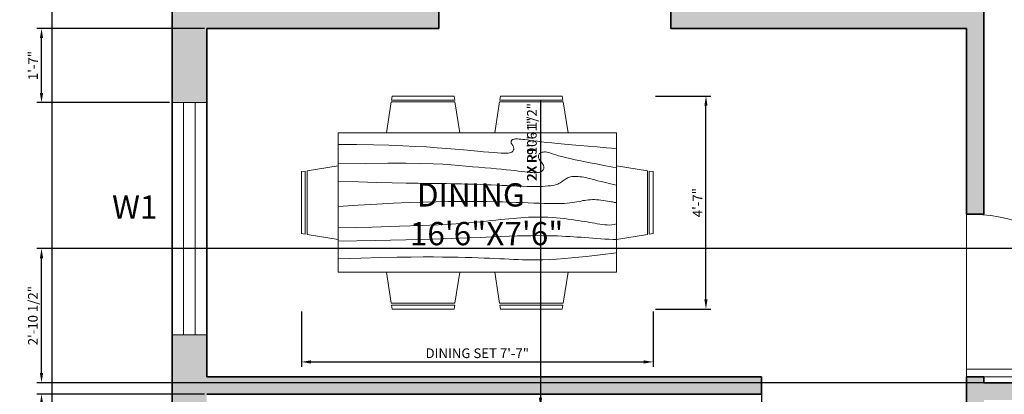
# Model space of a CAD drawing. Units: inches. Extents: x 5030 to 5465, y 5339 to 6047.
# Tile 3 of 5: x 5030 to 5285, y 5771 to 5867. Entities that reach past the tile are written whole.
import ezdxf

# ---------------------------------------------------------------- set-up
doc = ezdxf.new("R2010")
doc.units = ezdxf.units.IN
for name, color, linetype, lineweight in [('A-ANNO-DIMS', 2, 'Continuous', 18), ('A-ANNO-TEXT', 7, 'Continuous', 18), ('A-AREA-IDEN', 7, 'Continuous', 25), ('A-DOOR', 3, 'Continuous', 18), ('A-FURN', 8, 'Continuous', 18), ('A-GLAZ', 4, 'Continuous', 18), ('A-WALL', 7, 'Continuous', 35)]:
    doc.layers.add(name, color=color, linetype=linetype, lineweight=lineweight)
doc.layers.add('A-WALL-PATT', color=149, linetype='Continuous', lineweight=13, true_color=0x444546)
doc.styles.get("Standard").update_dxf_attribs({"font": 'arial.ttf'})
doc.dimstyles.new('ISO-25', dxfattribs={"dimtxt": 2.5, "dimasz": 2.5, "dimexe": 1.25, "dimexo": 0.625, "dimtad": 1, "dimlunit": 3, "dimtxsty": 'Standard', "dimcen": 2.5, "dimadec": 0, "dimazin": 0, "dimtfac": 1, "dimtmove": 0, "dimatfit": 3, "dimfxl": 1, "dimarcsym": 0})

# ---------------------------------------------------------------- blocks, each defined once
blk = doc.blocks.new('Dining Set - 36 x 72 in.')
for p, q in [((-22.2343, 26.00059), (-23.4847, 17.99762)), ((-22.2304, 26), (-5.7608, 26)), ((-22, 27.5), (-22.1562, 26.50042)), ((-5.8416, 26.5), (-22.1534, 26.5)), ((-22, 27.5), (-6, 27.5)), ((-5.8437, 26.49966), (-6, 27.5)), ((-4.5152, 17.99762), (-5.7655, 25.99926)), ((5.7657, 26.00059), (4.5153, 17.99762)), ((5.7696, 26), (22.2392, 26)), ((6, 27.5), (5.8438, 26.50042)), ((22.1584, 26.5), (5.8466, 26.5)), ((6, 27.5), (22, 27.5)), ((22.1563, 26.49966), (22, 27.5)), ((23.4848, 17.99762), (22.2345, 25.99926)), ((36, 18), (-36, 18)), ((-36, 18), (-36, -18)), ((36, -18), (36, 18)), ((-45.5, 8), (-44.5004, 8.15617)), ((-45.5, 8), (-45.5, -8)), ((-44.5, -8.15843), (-44.5, 8.15338)), ((-44.0006, 8.23428), (-35.9976, 9.48474)), ((-44, 8.23041), (-44, -8.23915)), ((44.0006, 8.23428), (35.9976, 9.48474)), ((44, 8.23041), (44, -8.23915)), ((44.5, -8.15843), (44.5, 8.15338)), ((45.5, 8), (44.5005, 8.15617)), ((45.5, 8), (45.5, -8)), ((-44.4997, -8.15631), (-45.5, -8)), ((-35.9976, -9.48476), (-43.9993, -8.2345)), ((35.9976, -9.48476), (43.9993, -8.2345)), ((44.4997, -8.15631), (45.5, -8)), ((-36, -18), (36, -18)), ((-22.2343, -26.0006), (-23.4847, -17.99762)), ((-4.5152, -17.99762), (-5.7655, -25.99928)), ((5.7657, -26.0006), (4.5153, -17.99762)), ((23.4848, -17.99762), (22.2345, -25.99928)), ((-22.2304, -26), (-5.7608, -26)), ((-22, -27.5), (-22.1562, -26.50044)), ((-5.8416, -26.5), (-22.1534, -26.5)), ((-22, -27.5), (-6, -27.5)), ((-5.8437, -26.49967), (-6, -27.5)), ((5.7696, -26), (22.2392, -26)), ((6, -27.5), (5.8438, -26.50044)), ((22.1584, -26.5), (5.8466, -26.5)), ((6, -27.5), (22, -27.5)), ((22.1563, -26.49967), (22, -27.5))]:
    blk.add_line(p, q)
for points in [[(-36, 15), (-31.1772, 14.97754), (-26.8079, 14.91406), (-22.8538, 14.81543), (-19.276, 14.6875), (-16.0362, 14.53613), (-13.0957, 14.36718), (-10.4159, 14.18652), (-7.9583, 14), (-5.6904, 13.81315), (-3.6035, 13.63021), (-1.6954, 13.45508), (0.0365, 13.29166), (1.5945, 13.14388), (2.9811, 13.01562), (4.1988, 12.9108), (5.25, 12.83333), (6.1393, 12.78613), (6.8802, 12.76823), (7.4883, 12.77767), (7.9792, 12.8125), (8.3685, 12.87077), (8.6719, 12.95052), (8.9049, 13.0498), (9.0833, 13.16666), (9.2205, 13.29899), (9.3216, 13.44401), (9.3895, 13.59879), (9.4271, 13.76041), (9.4373, 13.92594), (9.4232, 14.09245), (9.3875, 14.257), (9.3333, 14.41666), (9.2638, 14.56917), (9.1836, 14.71484), (9.0975, 14.85465), (9.0104, 14.98958), (8.9272, 15.1206), (8.8529, 15.2487), (8.7922, 15.37483), (8.75, 15.5), (8.7305, 15.62467), (8.7344, 15.74739), (8.7617, 15.86621), (8.8125, 15.97916), (8.8867, 16.08431), (8.9844, 16.17968), (9.1055, 16.26334), (9.25, 16.33333), (9.4189, 16.38802), (9.6172, 16.42708), (9.8506, 16.45052), (10.125, 16.45833), (10.4463, 16.45052), (10.8203, 16.42708), (11.2529, 16.38802), (11.75, 16.33333), (12.3184, 16.26318), (12.9694, 16.17838), (13.7151, 16.07991), (14.5677, 15.96875), (15.5395, 15.84586), (16.6426, 15.71224), (17.8893, 15.56884), (19.2917, 15.41666), (20.859, 15.25667), (22.5879, 15.08984), (24.4721, 14.91715), (26.5052, 14.73958), (28.6809, 14.5581), (30.9929, 14.3737), (33.4347, 14.18733), (36, 14)], [(-36, 10), (-28.9766, 10.14274), (-23.1725, 10.20442), (-18.4241, 10.19775), (-14.5677, 10.13541), (-11.4399, 10.03011), (-8.877, 9.89453), (-6.7154, 9.74137), (-4.7917, 9.58333), (-2.9698, 9.43082), (-1.2246, 9.28515), (0.4415, 9.14534), (2.026, 9.01041), (3.5266, 8.87939), (4.9408, 8.7513), (6.266, 8.62516), (7.5, 8.5), (8.6411, 8.37549), (9.6914, 8.2539), (10.6538, 8.13818), (11.5312, 8.03125), (12.3267, 7.93603), (13.043, 7.85547), (13.6831, 7.79248), (14.25, 7.75), (14.7471, 7.7303), (15.1797, 7.73307), (15.5537, 7.75732), (15.875, 7.80208), (16.1494, 7.86637), (16.3828, 7.94922), (16.5811, 8.04964), (16.75, 8.16666), (16.8944, 8.29915), (17.0143, 8.44531), (17.1089, 8.60319), (17.1771, 8.77083), (17.218, 8.94629), (17.2305, 9.1276), (17.2137, 9.31282), (17.1667, 9.5), (17.0895, 9.6875), (16.987, 9.875), (16.8649, 10.0625), (16.7292, 10.25), (16.5856, 10.4375), (16.4401, 10.625), (16.2985, 10.8125), (16.1667, 11), (16.05, 11.18733), (15.9518, 11.3737), (15.8752, 11.5581), (15.8229, 11.73958), (15.798, 11.91715), (15.8034, 12.08984), (15.842, 12.25667), (15.9167, 12.41666), (16.0295, 12.56836), (16.1784, 12.70833), (16.3605, 12.83268), (16.5729, 12.9375), (16.8127, 13.01888), (17.0768, 13.07291), (17.3625, 13.0957), (17.6667, 13.08333), (17.9894, 13.03312), (18.3418, 12.94726), (18.7382, 12.82918), (19.1927, 12.68229), (19.7195, 12.51001), (20.3327, 12.31575), (21.0465, 12.10294), (21.875, 11.875), (22.8357, 11.63354), (23.959, 11.37304), (25.2786, 11.08618), (26.8282, 10.76562), (28.6414, 10.40405), (30.752, 9.99414), (33.1936, 9.52856), (36, 9)], [(-36, 5.5), (-30.7157, 5.3348), (-26.069, 5.20963), (-21.9946, 5.11767), (-18.4271, 5.05208), (-15.3009, 5.00602), (-12.5508, 4.97265), (-10.1112, 4.94515), (-7.9167, 4.91666), (-5.909, 4.88167), (-4.0586, 4.83984), (-2.3429, 4.79215), (-0.7396, 4.73958), (0.7739, 4.6831), (2.22, 4.6237), (3.6213, 4.56233), (5, 4.5), (6.373, 4.43782), (7.7344, 4.3776), (9.0723, 4.32129), (10.375, 4.27083), (11.6309, 4.22819), (12.8281, 4.19531), (13.9551, 4.17415), (15, 4.16666), (15.954, 4.17448), (16.819, 4.19791), (17.6001, 4.23698), (18.3021, 4.29166), (18.9299, 4.36198), (19.4883, 4.44791), (19.9823, 4.54948), (20.4167, 4.66666), (20.7969, 4.79899), (21.1302, 4.94401), (21.4245, 5.09879), (21.6875, 5.26041), (21.9271, 5.42594), (22.1511, 5.59245), (22.3672, 5.757), (22.5834, 5.91666), (22.8065, 6.06868), (23.0404, 6.21093), (23.2879, 6.34147), (23.5521, 6.45833), (23.8358, 6.55957), (24.142, 6.64323), (24.4735, 6.70735), (24.8334, 6.75), (25.2235, 6.76969), (25.642, 6.76692), (26.0858, 6.74267), (26.5521, 6.69791), (27.0379, 6.63362), (27.5404, 6.55078), (28.0565, 6.45036), (28.5834, 6.33333), (29.1242, 6.19987), (29.7071, 6.04687), (30.3661, 5.87044), (31.1354, 5.66666), (32.0493, 5.43164), (33.142, 5.16146), (34.4475, 4.85221), (36, 4.5)], [(-36, -1), (-30.7915, -0.6591), (-26.0195, -0.38216), (-21.6519, -0.16284), (-17.6563, 0.00521), (-14.0005, 0.12833), (-10.6523, 0.21289), (-7.5796, 0.26522), (-4.75, 0.29166), (-2.134, 0.29793), (0.2878, 0.28711), (2.5317, 0.26163), (4.6146, 0.22396), (6.5529, 0.17651), (8.3633, 0.12174), (10.0623, 0.06209), (11.6667, 0), (13.1899, -0.06201), (14.6341, -0.1211), (15.9982, -0.17432), (17.2813, -0.21875), (18.4823, -0.25147), (19.6003, -0.26953), (20.6343, -0.27002), (21.5834, -0.25), (22.4481, -0.20768), (23.2357, -0.14584), (23.9549, -0.06836), (24.6146, 0.02083), (25.2235, 0.11784), (25.7904, 0.21875), (26.3241, 0.31966), (26.8334, 0.41666), (27.3265, 0.50618), (27.8099, 0.58593), (28.2894, 0.65397), (28.7709, 0.70833), (29.2601, 0.74707), (29.763, 0.76823), (30.2855, 0.76985), (30.8334, 0.75), (31.4088, 0.70784), (31.9994, 0.64713), (32.589, 0.57275), (33.1615, 0.48958), (33.7008, 0.4025), (34.1908, 0.3164), (34.6153, 0.23616), (34.9584, 0.16666), (35.2099, 0.11165), (35.3848, 0.07031), (35.504, 0.04069), (35.5886, 0.02083), (35.6594, 0.00879), (35.7377, 0.0026), (35.8442, 0.00032), (36, 0)], [(-36, -6.5), (-27.1843, -6.31267), (-20.084, -6.1263), (-14.469, -5.9419), (-10.1094, -5.76042), (-6.7752, -5.58285), (-4.2363, -5.41016), (-2.2629, -5.24333), (-0.625, -5.08334), (0.8708, -4.93099), (2.2715, -4.78646), (3.5872, -4.64974), (4.8281, -4.52084), (6.0046, -4.39974), (7.127, -4.28646), (8.2053, -4.18099), (9.25, -4.08334), (10.2705, -3.99382), (11.2734, -3.91407), (12.2647, -3.84603), (13.25, -3.79167), (14.2354, -3.75293), (15.2266, -3.73177), (16.2295, -3.73015), (17.25, -3.75), (18.2912, -3.79248), (19.3451, -3.85547), (20.4009, -3.93604), (21.4479, -4.03125), (22.4754, -4.13819), (23.4727, -4.25391), (24.4289, -4.37549), (25.3334, -4.5), (26.1785, -4.62492), (26.9694, -4.74935), (27.7145, -4.87281), (28.4219, -4.99479), (29.1, -5.11483), (29.7572, -5.23242), (30.4016, -5.34709), (31.0417, -5.45834), (31.6837, -5.56437), (32.3262, -5.65821), (32.9658, -5.73153), (33.599, -5.77604), (34.2224, -5.78345), (34.8327, -5.74545), (35.4264, -5.65373), (36, -5.5)], [(-36, -10), (-26.4022, -9.81299), (-18.4675, -9.62891), (-11.9839, -9.45069), (-6.7396, -9.28125), (-2.5226, -9.12354), (0.8789, -8.98047), (3.6769, -8.85498), (6.0833, -8.75), (8.2767, -8.66765), (10.3021, -8.60677), (12.1712, -8.56543), (13.8958, -8.54167), (15.4876, -8.53353), (16.9583, -8.53907), (18.3197, -8.55632), (19.5834, -8.58334), (20.7616, -8.61841), (21.8685, -8.66081), (22.9188, -8.71004), (23.9271, -8.76563), (24.9081, -8.82707), (25.8763, -8.89388), (26.8465, -8.96558), (27.8334, -9.04167), (28.8474, -9.12118), (29.8828, -9.20117), (30.93, -9.27824), (31.9792, -9.34896), (33.0205, -9.40991), (34.0443, -9.45768), (35.0407, -9.48885), (36, -9.5)], [(-36, -14.5), (-30.0881, -14.33513), (-25.0332, -14.21224), (-20.7312, -14.12647), (-17.0781, -14.07292), (-13.97, -14.04671), (-11.3027, -14.04297), (-8.9724, -14.05681), (-6.875, -14.08334), (-4.9224, -14.11833), (-3.0905, -14.16016), (-1.3709, -14.20785), (0.2448, -14.26042), (1.7647, -14.3169), (3.1973, -14.3763), (4.5507, -14.43767), (5.8333, -14.5), (7.0554, -14.5621), (8.235, -14.62175), (9.3922, -14.67652), (10.5469, -14.72396), (11.7192, -14.76164), (12.929, -14.78711), (14.1965, -14.79794), (15.5417, -14.79167), (16.9933, -14.76424), (18.6152, -14.70508), (20.4804, -14.60197), (22.6615, -14.44271), (25.2312, -14.21509), (28.2624, -13.9069), (31.8277, -13.50594), (36, -13)]]:
    blk.add_lwpolyline(points)
blk = doc.blocks.new('*D8')
at = {"layer": 'A-ANNO-DIMS', "color": 0, "lineweight": -2, "transparency": 16777216}
for p, q in [((5068.62, 5971.96), (5036.91, 5971.96)), ((5038.16, 5969.46), (5038.16, 5377)), ((5068.62, 5374.5), (5036.91, 5374.5))]:
    blk.add_line(p, q, dxfattribs=at)
at = {"layer": 'A-ANNO-DIMS', "color": 0, "transparency": 16777216}
for points in [[(5037.74, 5969.46), (5038.58, 5969.46), (5038.16, 5971.96)], [(5037.74, 5377), (5038.58, 5377), (5038.16, 5374.5)]]:
    blk.add_solid(points, dxfattribs=at)
at = {"layer": 'Defpoints', "color": 0, "transparency": 16777216}
for p in [(5069.24, 5971.96), (5038.16, 5374.5), (5069.24, 5374.5)]:
    blk.add_point(p, dxfattribs=at)
at = {"layer": 'A-ANNO-DIMS', "color": 0, "transparency": 16777216, "insert": (5034.47, 5673.23), "char_height": 6, "attachment_point": 5, "rotation": 90}
blk.add_mtext('49\'-9.46"', dxfattribs=at)
blk = doc.blocks.new('WIN-60IN')
for p, q in [((0, 60), (9, 60)), ((3, 60), (3, 0)), ((6, 60), (6, 0)), ((0, 0), (9, 0))]:
    blk.add_line(p, q)
blk = doc.blocks.new('DOOR-SWING-42IN')
for p, q in [((0, 0), (0, 42)), ((0, 42), (2, 42)), ((2, 42), (2, 0)), ((2, 0), (0, 0))]:
    blk.add_line(p, q)
blk.add_arc((1, 1), 41.01, 358.6028, 91.3972)
blk = doc.blocks.new('*D27')
at = {"layer": 'A-ANNO-DIMS', "color": 0, "lineweight": -2, "transparency": 16777216}
for p, q in [((5102.7, 5791.89), (5102.7, 5777.61)), ((5193.7, 5791.89), (5193.7, 5777.61)), ((5105.2, 5778.86), (5191.2, 5778.86))]:
    blk.add_line(p, q, dxfattribs=at)
at = {"layer": 'A-ANNO-DIMS', "color": 0, "transparency": 16777216}
for points in [[(5105.2, 5779.28), (5105.2, 5778.44), (5102.7, 5778.86)], [(5191.2, 5779.28), (5191.2, 5778.44), (5193.7, 5778.86)]]:
    blk.add_solid(points, dxfattribs=at)
at = {"layer": 'Defpoints', "color": 0, "transparency": 16777216}
for p in [(5102.7, 5792.51), (5193.7, 5792.51), (5193.7, 5778.86)]:
    blk.add_point(p, dxfattribs=at)
at = {"layer": 'A-ANNO-DIMS', "color": 0, "transparency": 16777216, "insert": (5148.2, 5780.78), "char_height": 2.5, "attachment_point": 5}
blk.add_mtext('DINING SET 7\'-7"', dxfattribs=at)
blk = doc.blocks.new('*D28')
at = {"layer": 'A-ANNO-DIMS', "color": 0, "lineweight": -2, "transparency": 16777216}
for p, q in [((5194.32, 5847.51), (5208.6, 5847.51)), ((5207.35, 5795.01), (5207.35, 5845.01)), ((5194.32, 5792.51), (5208.6, 5792.51))]:
    blk.add_line(p, q, dxfattribs=at)
at = {"layer": 'A-ANNO-DIMS', "color": 0, "transparency": 16777216}
for points in [[(5206.93, 5845.01), (5207.76, 5845.01), (5207.35, 5847.51)], [(5206.93, 5795.01), (5207.76, 5795.01), (5207.35, 5792.51)]]:
    blk.add_solid(points, dxfattribs=at)
at = {"layer": 'Defpoints', "color": 0, "transparency": 16777216}
for p in [(5193.7, 5847.51), (5207.35, 5847.51), (5193.7, 5792.51)]:
    blk.add_point(p, dxfattribs=at)
at = {"layer": 'A-ANNO-DIMS', "color": 0, "transparency": 16777216, "insert": (5205.47, 5820.01), "char_height": 2.5, "attachment_point": 5, "rotation": 90}
blk.add_mtext('4\'-7"', dxfattribs=at)
blk = doc.blocks.new('*D47')
at = {"layer": 'A-ANNO-DIMS', "color": 0, "lineweight": -2, "transparency": 16777216}
for p, q in [((5077.62, 5865), (5034.24, 5865)), ((5035.49, 5848.34), (5035.49, 5862.5)), ((5068.62, 5845.84), (5034.24, 5845.84))]:
    blk.add_line(p, q, dxfattribs=at)
at = {"layer": 'A-ANNO-DIMS', "color": 0, "transparency": 16777216}
for points in [[(5035.07, 5862.5), (5035.91, 5862.5), (5035.49, 5865)], [(5035.07, 5848.34), (5035.91, 5848.34), (5035.49, 5845.84)]]:
    blk.add_solid(points, dxfattribs=at)
at = {"layer": 'Defpoints', "color": 0, "transparency": 16777216}
for p in [(5035.49, 5865), (5078.24, 5865), (5069.24, 5845.84)]:
    blk.add_point(p, dxfattribs=at)
at = {"layer": 'A-ANNO-DIMS', "color": 0, "transparency": 16777216, "insert": (5033.61, 5855.42), "char_height": 2.5, "attachment_point": 5, "rotation": 90}
blk.add_mtext('1\'-7"', dxfattribs=at)
blk = doc.blocks.new('*D48')
at = {"layer": 'A-ANNO-DIMS', "color": 0, "lineweight": -2, "transparency": 16777216}
for p, q in [((5077.62, 5770.5), (5034.24, 5770.5)), ((5035.49, 5745.65), (5035.49, 5768)), ((5068.62, 5743.15), (5034.24, 5743.15))]:
    blk.add_line(p, q, dxfattribs=at)
at = {"layer": 'A-ANNO-DIMS', "color": 0, "transparency": 16777216}
for points in [[(5035.07, 5768), (5035.91, 5768), (5035.49, 5770.5)], [(5035.07, 5745.65), (5035.91, 5745.65), (5035.49, 5743.15)]]:
    blk.add_solid(points, dxfattribs=at)
at = {"layer": 'Defpoints', "color": 0, "transparency": 16777216}
for p in [(5035.49, 5770.5), (5078.24, 5770.5), (5069.24, 5743.15)]:
    blk.add_point(p, dxfattribs=at)
at = {"layer": 'A-ANNO-DIMS', "color": 0, "transparency": 16777216, "insert": (5033.57, 5756.83), "char_height": 2.5, "attachment_point": 5, "rotation": 90}
blk.add_mtext('2\'-3 1/2"', dxfattribs=at)
blk = doc.blocks.new('*D54')
at = {"layer": 'A-ANNO-DIMS', "color": 0, "lineweight": -2, "transparency": 16777216}
for p, q in [((5138.24, 5870.13), (5138.24, 6009.5)), ((5140.74, 6008.25), (5195.74, 6008.25)), ((5198.24, 5865.63), (5198.24, 6009.5))]:
    blk.add_line(p, q, dxfattribs=at)
at = {"layer": 'A-ANNO-DIMS', "color": 0, "transparency": 16777216}
for points in [[(5140.74, 6008.67), (5140.74, 6007.84), (5138.24, 6008.25)], [(5195.74, 6008.67), (5195.74, 6007.84), (5198.24, 6008.25)]]:
    blk.add_solid(points, dxfattribs=at)
at = {"layer": 'Defpoints', "color": 0, "transparency": 16777216}
for p in [(5198.24, 6008.25), (5138.24, 5869.5), (5198.24, 5865)]:
    blk.add_point(p, dxfattribs=at)
at = {"layer": 'A-ANNO-DIMS', "color": 0, "transparency": 16777216, "insert": (5168.24, 6010.15), "char_height": 2.5, "attachment_point": 5}
blk.add_mtext('5\'-0"', dxfattribs=at)
blk = doc.blocks.new('*D55')
at = {"layer": 'A-ANNO-DIMS', "color": 0, "lineweight": -2, "transparency": 16777216}
for p, q in [((5221.75, 5774.38), (5221.75, 5339.5)), ((5274.74, 5774.38), (5274.74, 5339.5)), ((5224.25, 5340.75), (5272.24, 5340.75))]:
    blk.add_line(p, q, dxfattribs=at)
at = {"layer": 'A-ANNO-DIMS', "color": 0, "transparency": 16777216}
for points in [[(5224.25, 5341.17), (5224.25, 5340.34), (5221.75, 5340.75)], [(5272.24, 5341.17), (5272.24, 5340.34), (5274.74, 5340.75)]]:
    blk.add_solid(points, dxfattribs=at)
at = {"layer": 'Defpoints', "color": 0, "transparency": 16777216}
for p in [(5221.75, 5775), (5274.74, 5775), (5274.74, 5340.75)]:
    blk.add_point(p, dxfattribs=at)
at = {"layer": 'A-ANNO-DIMS', "color": 0, "transparency": 16777216, "insert": (5248.24, 5342.65), "char_height": 2.5, "attachment_point": 5}
blk.add_mtext('4\'-5"', dxfattribs=at)
blk = doc.blocks.new('*D57')
at = {"layer": 'A-ANNO-DIMS', "color": 0, "lineweight": -2, "transparency": 16777216}
for p, q in [((5359.62, 5808.14), (5034.24, 5808.14)), ((5035.49, 5776), (5035.49, 5805.64)), ((5359.62, 5773.5), (5034.24, 5773.5))]:
    blk.add_line(p, q, dxfattribs=at)
at = {"layer": 'A-ANNO-DIMS', "color": 0, "transparency": 16777216}
for points in [[(5035.07, 5805.64), (5035.91, 5805.64), (5035.49, 5808.14)], [(5035.07, 5776), (5035.91, 5776), (5035.49, 5773.5)]]:
    blk.add_solid(points, dxfattribs=at)
at = {"layer": 'Defpoints', "color": 0, "transparency": 16777216}
for p in [(5035.49, 5808.14), (5360.24, 5808.14), (5360.24, 5773.5)]:
    blk.add_point(p, dxfattribs=at)
at = {"layer": 'A-ANNO-DIMS', "color": 0, "transparency": 16777216, "insert": (5033.57, 5790.82), "char_height": 2.5, "attachment_point": 5, "rotation": 90}
blk.add_mtext('2\'-10 1/2"', dxfattribs=at)
blk = doc.blocks.new('*D66')
at = {"layer": 'A-ANNO-DIMS', "color": 0, "lineweight": -2, "transparency": 16777216}
for p, q in [((5164.56, 5842.64), (5164.56, 5763.6)), ((5164.56, 5639.91), (5164.56, 5761.1))]:
    blk.add_line(p, q, dxfattribs=at)
at = {"layer": 'A-ANNO-DIMS', "color": 0, "transparency": 16777216}
blk.add_solid([(5164.14, 5763.6), (5164.98, 5763.6), (5164.56, 5761.1)], dxfattribs=at)
at = {"layer": 'Defpoints', "color": 0, "transparency": 16777216}
for p in [(5164.56, 5761.1), (5164.56, 5639.91)]:
    blk.add_point(p, dxfattribs=at)
at = {"layer": 'A-ANNO-DIMS', "color": 0, "transparency": 16777216, "insert": (5162.66, 5833.82), "char_height": 2.5, "attachment_point": 5, "rotation": 89.9998}
blk.add_mtext('2X R10\'-1"', dxfattribs=at)
blk = doc.blocks.new('*D67')
at = {"layer": 'A-ANNO-DIMS', "color": 0, "lineweight": -2, "transparency": 16777216}
for p, q in [((5164.56, 5846.42), (5164.56, 5769.6)), ((5164.56, 5652.85), (5164.56, 5767.1))]:
    blk.add_line(p, q, dxfattribs=at)
at = {"layer": 'A-ANNO-DIMS', "color": 0, "transparency": 16777216}
blk.add_solid([(5164.14, 5769.6), (5164.98, 5769.6), (5164.56, 5767.1)], dxfattribs=at)
at = {"layer": 'Defpoints', "color": 0, "transparency": 16777216}
for p in [(5164.56, 5767.1), (5164.56, 5652.85)]:
    blk.add_point(p, dxfattribs=at)
at = {"layer": 'A-ANNO-DIMS', "color": 0, "transparency": 16777216, "insert": (5162.64, 5835.65), "char_height": 2.5, "attachment_point": 5, "rotation": 89.9998}
blk.add_mtext('2X R9\'-6 1/2"', dxfattribs=at)

msp = doc.modelspace()

# ---------------------------------------------------------------- hatches: boundary and pattern name
at = {"layer": 'A-WALL-PATT'}
h = msp.add_hatch(color=256, dxfattribs=at)
h.dxf.hatch_style = 1
h.paths.add_polyline_path([(5227.999, 5974.503), (5069.24, 5974.503), (5069.24, 5942.38), (5078.24, 5942.38), (5078.24, 5965.503), (5198.24, 5965.503), (5198.24, 5916.003), (5274.74, 5916.003), (5274.74, 5869.503), (5202.74, 5869.503), (5202.74, 5898.003), (5198.24, 5898.003), (5198.24, 5865.003), (5274.74, 5865.003), (5274.74, 5817.003, -0.0121933), (5276.74, 5817.003), (5279.24, 5817.003), (5279.24, 5947.503, -0.0293864), (5277.24, 5947.503), (5274.74, 5947.503), (5274.74, 5920.503), (5202.74, 5920.503), (5202.74, 5965.503), (5227.999, 5965.503)])
h.paths.add_polyline_path([(5078.24, 5894.38), (5069.24, 5894.38), (5069.24, 5845.837), (5078.24, 5845.837), (5078.24, 5865.003), (5138.24, 5865.003), (5138.24, 5869.503), (5078.24, 5869.503)], flags=17)
h.paths.add_polyline_path([(5316.341, 5974.503), (5251.999, 5974.503), (5251.999, 5965.503), (5279.24, 5965.503), (5316.341, 5965.503)])
h.paths.add_polyline_path([(5429.24, 5974.503), (5376.341, 5974.503), (5376.341, 5965.503), (5420.24, 5965.503), (5420.24, 5904.986), (5429.24, 5904.986)])
h.paths.add_polyline_path([(5429.24, 5844.986), (5420.24, 5844.986), (5420.24, 5773.503), (5279.24, 5773.503), (5279.24, 5775.003), (5274.74, 5775.003), (5274.74, 5644.503), (5279.24, 5644.503), (5279.24, 5686.503), (5279.24, 5769.003), (5420.24, 5769.003), (5420.24, 5738.095), (5429.24, 5738.095)])
h.paths.add_polyline_path([(5429.24, 5678.095), (5420.24, 5678.095), (5420.24, 5649.003), (5321.24, 5649.003), (5321.24, 5646.503, -0.0121933), (5321.24, 5644.503), (5343.74, 5644.503), (5343.74, 5614.503, -0.0293864), (5345.74, 5614.503), (5348.24, 5614.503), (5348.24, 5644.503), (5420.24, 5644.503), (5420.24, 5636.807), (5429.24, 5636.807)])
h.paths.add_polyline_path([(5429.24, 5612.807), (5420.24, 5612.807), (5420.24, 5596.503), (5321.24, 5596.503, -0.0121933), (5321.24, 5594.503), (5321.24, 5592.003), (5420.24, 5592.003), (5420.24, 5566.431), (5429.24, 5566.431)])
h.paths.add_polyline_path([(5429.24, 5506.431), (5420.24, 5506.431), (5420.24, 5472.003), (5279.24, 5472.003), (5279.24, 5596.503), (5126.24, 5596.503), (5126.24, 5589.503, -0.0106371), (5126.24, 5587.503), (5274.74, 5587.503), (5274.74, 5468.003), (5420.24, 5468.003), (5420.24, 5452.536), (5429.24, 5452.536)])
h.paths.add_polyline_path([(5429.24, 5392.536), (5420.24, 5392.536), (5420.24, 5383.503), (5274.74, 5383.503), (5274.74, 5374.503), (5429.24, 5374.503)])
h.paths.add_polyline_path([(5101.667, 5383.503), (5078.24, 5383.503), (5078.24, 5683.152), (5069.24, 5683.152), (5069.24, 5374.503), (5101.667, 5374.503)])
h.paths.add_polyline_path([(5078.24, 5770.503), (5221.745, 5770.503), (5221.745, 5775.003), (5078.24, 5775.003), (5078.24, 5785.837), (5069.24, 5785.837), (5069.24, 5743.152), (5078.24, 5743.152)])
h.paths.add_polyline_path([(5274.74, 5379.003), (5101.667, 5379.003), (5101.667, 5374.503), (5274.74, 5374.503)])

# ---------------------------------------------------------------- linework, layer by layer
at = {"layer": 'A-DOOR'}
msp.add_line((5274.74, 5777.003), (5274.74, 5817.003), dxfattribs=at)
at = {"layer": 'A-WALL'}
for p, q in [((5069.24, 5374.503), (5069.24, 5974.503)), ((5279.24, 5817.003), (5279.24, 5947.503)), ((5198.24, 5865.003), (5198.24, 5898.003)), ((5138.24, 5869.503), (5138.24, 5865.003)), ((5078.24, 5865.003), (5138.24, 5865.003)), ((5078.24, 5775.003), (5078.24, 5865.003)), ((5198.24, 5865.003), (5274.74, 5865.003)), ((5274.74, 5817.003), (5274.74, 5865.003)), ((5274.74, 5817.003), (5279.24, 5817.003)), ((5078.24, 5775.003), (5221.745, 5775.003)), ((5221.745, 5775.003), (5221.745, 5770.503)), ((5274.74, 5644.503), (5274.74, 5775.003)), ((5274.74, 5775.003), (5279.24, 5775.003)), ((5279.24, 5773.503), (5279.24, 5775.003)), ((5279.24, 5773.503), (5420.24, 5773.503)), ((5078.24, 5770.503), (5221.745, 5770.503))]:
    msp.add_line(p, q, dxfattribs=at)

# ---------------------------------------------------------------- block references
at = {"layer": 'A-DOOR', "extrusion": (0, 0, -1), "zscale": -1, "rotation": 90.00000000000831}
msp.add_blockref('DOOR-SWING-42IN', (-5274.74, 5775.003), dxfattribs=at)
at = {"layer": 'A-FURN'}
msp.add_blockref('Dining Set - 36 x 72 in.', (5148.198, 5820.011), dxfattribs=at)
at = {"layer": 'A-GLAZ'}
msp.add_blockref('WIN-60IN', (5069.24, 5785.837), dxfattribs=at)

# ---------------------------------------------------------------- texts
at = {"layer": 'A-ANNO-TEXT', "insert": (5053.75, 5821.85), "char_height": 6, "attachment_point": 1}
msp.add_mtext_dynamic_manual_height_columns('W1 ', width=54.21026, gutter_width=12.5, heights=[0], dxfattribs=at)
at = {"layer": 'A-AREA-IDEN', "insert": (5130.735, 5825.002), "char_height": 6, "attachment_point": 1}
msp.add_mtext_dynamic_manual_height_columns(' DINING{\\fTimes New Roman|b0|i0|c0|p18;\\P16\'6"X7\'6"}', width=54.21026, gutter_width=12.5, heights=[0], dxfattribs=at)

# ---------------------------------------------------------------- dimensions: what is measured, and where the dimension line sits
at = {"layer": 'A-ANNO-DIMS'}
for base, p1, p2, picture, middle in [((5198.24, 6008.253), (5138.24, 5869.503), (5198.24, 5865.003), '*D54', (5168.24, 6010.155)), ((5274.74, 5340.753), (5221.745, 5775.003), (5274.74, 5775.003), '*D55', (5248.243, 5342.649))]:
    dim = msp.add_linear_dim(base=base, p1=p1, p2=p2, dimstyle='ISO-25', override={"dimdec": 1, "dimlfac": 1, "dimrnd": 0, "dimzin": 1, "dimdsep": 46, "dimlunit": 4, "dimfrac": 2}, dxfattribs=at)
    dim.commit()
    dim.dimension.update_dxf_attribs({"geometry": picture, "text_midpoint": middle})
for base, p1, p2, override, picture, middle in [((5038.161, 5374.503), (5069.24, 5971.965), (5069.24, 5374.503), {"dimtxt": 6, "dimclrd": 0, "dimclre": 0, "dimclrt": 0}, '*D8', (5034.472, 5673.234)), ((5035.49, 5865.003), (5069.24, 5845.837), (5078.24, 5865.003), {"dimdec": 1, "dimlfac": 1, "dimrnd": 0, "dimzin": 1, "dimdsep": 46, "dimlunit": 4, "dimfrac": 2}, '*D47', (5033.61, 5855.42)), ((5207.348, 5847.511), (5193.698, 5792.511), (5193.698, 5847.511), {"dimdec": 1, "dimlfac": 1, "dimrnd": 0, "dimzin": 1, "dimdsep": 46, "dimlunit": 4, "dimfrac": 2}, '*D28', (5205.473, 5820.011)), ((5035.49, 5808.145), (5360.24, 5773.503), (5360.24, 5808.145), {"dimdec": 1, "dimlfac": 1, "dimrnd": 0, "dimzin": 1, "dimdsep": 46, "dimlunit": 4, "dimfrac": 2}, '*D57', (5033.573, 5790.824)), ((5035.49, 5770.503), (5069.24, 5743.152), (5078.24, 5770.503), {"dimdec": 1, "dimlfac": 1, "dimrnd": 0, "dimzin": 1, "dimdsep": 46, "dimlunit": 4, "dimfrac": 2}, '*D48', (5033.572, 5756.828))]:
    dim = msp.add_linear_dim(base=base, p1=p1, p2=p2, angle=90, dimstyle='ISO-25', override=override, dxfattribs=at)
    dim.commit()
    dim.dimension.update_dxf_attribs({"geometry": picture, "text_midpoint": middle})
for center, mpoint, picture, middle in [((5164.55865, 5652.852134), (5164.559, 5767.102134), '*D67', (5164.55921, 5835.652134)), ((5164.559, 5639.905), (5164.559, 5761.102), '*D66', (5164.559, 5833.82))]:
    dim = msp.add_radius_dim(center=center, mpoint=mpoint, text='2X <>', dimstyle='ISO-25', override={"dimdec": 1, "dimlfac": 1, "dimrnd": 0, "dimzin": 1, "dimdsep": 46, "dimlunit": 4, "dimfrac": 2}, dxfattribs=at)
    dim.commit()
    dim.dimension.update_dxf_attribs({"geometry": picture, "text_midpoint": middle, "dimtype": 164})
dim = msp.add_linear_dim(base=(5193.698, 5778.861), p1=(5102.698, 5792.511), p2=(5193.698, 5792.511), text='DINING SET <>', dimstyle='ISO-25', override={"dimdec": 1, "dimlfac": 1, "dimrnd": 0, "dimzin": 1, "dimdsep": 46, "dimlunit": 4, "dimfrac": 2}, dxfattribs=at)
dim.commit()
dim.dimension.update_dxf_attribs({"geometry": '*D27', "text_midpoint": (5148.198, 5780.778)})

doc.saveas('drawing.dxf')
